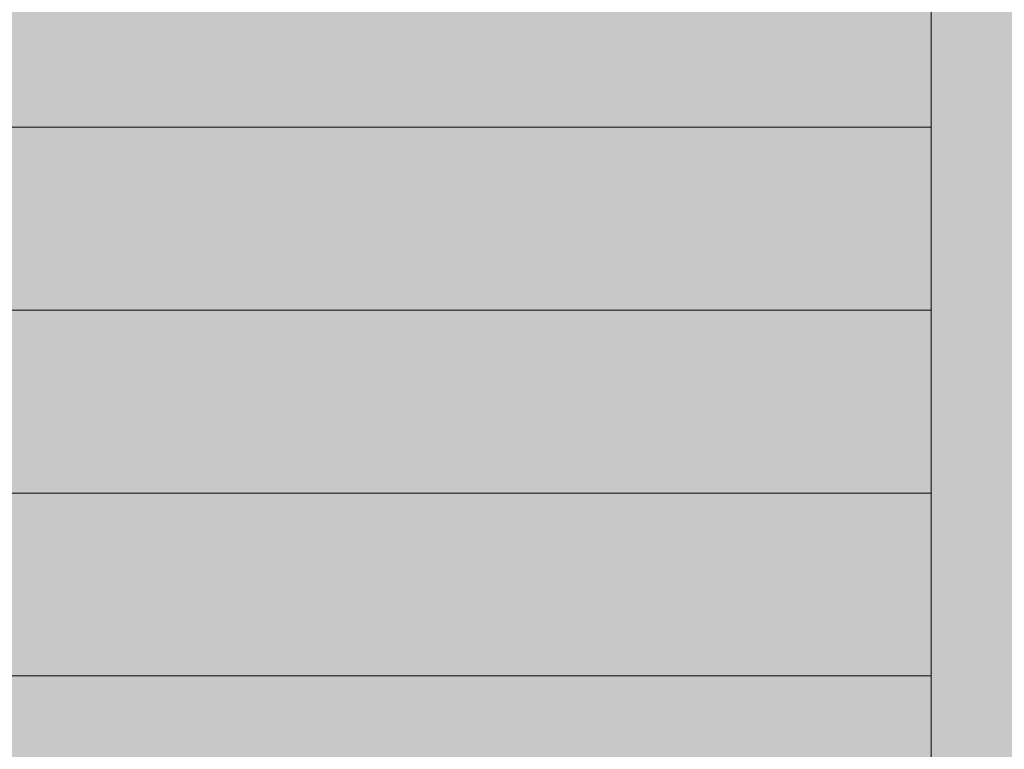
# Model space of a CAD drawing. Units: inches. Extents: x 1704 to 6393, y -157 to 1172.
# Tile 103 of 122: x 2627 to 2667, y 972 to 1002. Entities that reach past the tile are written whole.
import ezdxf

# ---------------------------------------------------------------- set-up
doc = ezdxf.new("R2010")
doc.units = ezdxf.units.IN
doc.header["$MEASUREMENT"] = 0
for name, color, linetype, lineweight in [('A-ANNO-DIMS', 7, 'Continuous', 13), ('L-DECK-PLNK-PATT', 250, 'Continuous', 13), ('L-HRDS', 8, 'Continuous', 18)]:
    doc.layers.add(name, color=color, linetype=linetype, lineweight=lineweight)
doc.layers.add('L-DECK-PATT', color=35, linetype='Continuous', lineweight=13, true_color=0xa6725b)
doc.layers.add('L-HRDS-PATT', color=9, linetype='Continuous', lineweight=13, true_color=0xc5c1ba)
doc.styles.get("Standard").update_dxf_attribs({"font": 'arial.ttf'})
doc.dimstyles.get("Standard").update_dxf_attribs({"dimtxt": 6, "dimasz": 2, "dimexe": 0.18, "dimexo": 0.0625, "dimgap": 0.09, "dimtad": 0, "dimtih": 1, "dimtoh": 1, "dimdec": 1, "dimzin": 0, "dimdsep": 46, "dimlunit": 3, "dimtxsty": 'Standard', "dimblk": 'ARCHTICK', "dimcen": 0.09, "dimadec": 0, "dimazin": 0, "dimtfac": 1, "dimtdec": 1, "dimtofl": 0, "dimtmove": 0, "dimatfit": 3, "dimfxl": 1, "dimtolj": 1, "dimtzin": 0, "dimarcsym": 0})

# ---------------------------------------------------------------- blocks, each defined once
blk = doc.blocks.new('_ArchTick')
at = {"color": 0, "linetype": 'ByBlock', "const_width": 0.15}
blk.add_lwpolyline([(-0.5, -0.5), (0.5, 0.5)], dxfattribs=at)
blk = doc.blocks.new('*D95')
at = {"layer": 'A-ANNO-DIMS', "color": 0, "lineweight": -2, "transparency": 16777216}
for p, q in [((2605.349, 895.275), (2605.349, 1105.287)), ((2605.349, 1105.107), (2657.907, 1105.107)), ((2723.349, 1105.107), (2670.791, 1105.107)), ((2723.349, 895.275), (2723.349, 1105.287))]:
    blk.add_line(p, q, dxfattribs=at)
at = {"layer": 'Defpoints', "color": 0, "lineweight": -3, "transparency": 16777216}
for p in [(2723.349, 1105.107), (2605.349, 895.213), (2723.349, 895.213)]:
    blk.add_point(p, dxfattribs=at)
at = {"layer": 'A-ANNO-DIMS', "color": 0, "lineweight": -2, "transparency": 16777216, "xscale": 2, "yscale": 2, "zscale": 2, "rotation": 180}
blk.add_blockref('_ArchTick', (2605.349, 1105.107), dxfattribs=at)
at = {"layer": 'A-ANNO-DIMS', "color": 0, "lineweight": -2, "transparency": 16777216, "xscale": 2, "yscale": 2, "zscale": 2}
blk.add_blockref('_ArchTick', (2723.349, 1105.107), dxfattribs=at)
at = {"layer": 'A-ANNO-DIMS', "color": 0, "transparency": 16777216, "insert": (2664.349, 1105.107), "char_height": 6, "attachment_point": 5}
blk.add_mtext('\\A1;118', dxfattribs=at)

msp = doc.modelspace()

# ---------------------------------------------------------------- hatches: boundary and pattern name
at = {"layer": 'L-DECK-PATT', "transparency": 33554544}
h = msp.add_hatch(color=256, dxfattribs=at)
h.dxf.hatch_style = 1
h.paths.add_polyline_path([(2329.589, 1033.213), (2065.589, 1033.213), (2065.589, 895.213), (2167.349, 895.213), (2263.349, 895.213), (2263.349, 903.213), (2273.349, 903.213), (2273.349, 895.213), (2329.589, 895.213)])
h.paths.add_polyline_path([(2664.349, 1033.213), (2333.589, 1033.213), (2333.589, 895.213), (2465.349, 895.213), (2469.181, 895.213), (2470.482, 895.213), (2508.215, 895.213), (2509.516, 895.213), (2513.349, 895.213), (2533.349, 895.213), (2581.349, 895.213), (2605.349, 895.213), (2664.349, 895.213)])
h.paths.add_polyline_path([(2333.589, 1033.213), (2329.589, 1033.213), (2329.589, 895.213), (2333.589, 895.213)])
at = {"layer": 'L-DECK-PLNK-PATT'}
h = msp.add_hatch(dxfattribs=at)
h.set_pattern_fill('LINE', color=256, scale=60)
h.paths.add_polyline_path([(2329.589, 1033.213), (2065.589, 1033.213), (2065.589, 895.213), (2167.349, 895.213), (2263.349, 895.213), (2263.349, 903.213), (2273.349, 903.213), (2273.349, 895.213), (2329.589, 895.213)])
h.paths.add_polyline_path([(2664.349, 1033.213), (2333.589, 1033.213), (2333.589, 895.213), (2465.349, 895.213), (2469.181, 895.213), (2470.482, 895.213), (2508.215, 895.213), (2509.516, 895.213), (2513.349, 895.213), (2533.349, 895.213), (2581.349, 895.213), (2605.349, 895.213), (2664.349, 895.213)])
h.paths.add_polyline_path([(2333.589, 1033.213), (2329.589, 1033.213), (2329.589, 895.213), (2333.589, 895.213)])
at = {"layer": 'L-HRDS-PATT', "transparency": 33554661}
h = msp.add_hatch(color=256, dxfattribs=at)
h.dxf.hatch_style = 1
h.paths.add_polyline_path([(2719.349, 1033.213), (2664.349, 1033.213), (2664.349, 895.213), (2719.349, 895.213)])
h.paths.add_polyline_path([(2719.349, 895.213), (2664.349, 895.213), (2605.349, 895.213), (2605.349, 872.213), (2719.349, 872.213)])
h.paths.add_polyline_path([(2719.349, 872.213), (2605.349, 872.213), (2605.349, 854.213), (2601.349, 854.213, -0.121066), (2618.034, 850.113), (2618.05, 850.14), (2619.349, 849.39), (2601.349, 818.213), (2605.349, 818.213), (2605.349, 794.213), (2605.349, 754.213), (2631.349, 754.213), (2631.349, 716.213), (2719.349, 716.213)])

# ---------------------------------------------------------------- linework, layer by layer
at = {"layer": 'L-HRDS'}
msp.add_line((2664.349, 895.213), (2664.349, 1033.213), dxfattribs=at)

# ---------------------------------------------------------------- dimensions: what is measured, and where the dimension line sits
at = {"layer": 'A-ANNO-DIMS'}
dim = msp.add_linear_dim(base=(2723.349, 1105.107), p1=(2605.349, 895.213), p2=(2723.349, 895.213), dimstyle='Standard', override={"dimdec": 0, "dimlfac": 1, "dimrnd": 0, "dimzin": 0, "dimdsep": 46, "dimlunit": 2}, dxfattribs=at)
dim.commit()
dim.dimension.update_dxf_attribs({"geometry": '*D95', "text_midpoint": (2664.349, 1105.107)})

doc.saveas('drawing.dxf')
